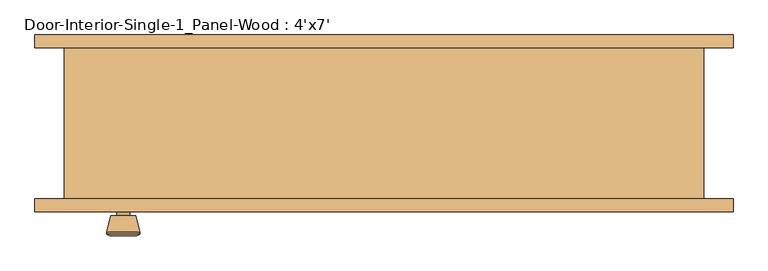
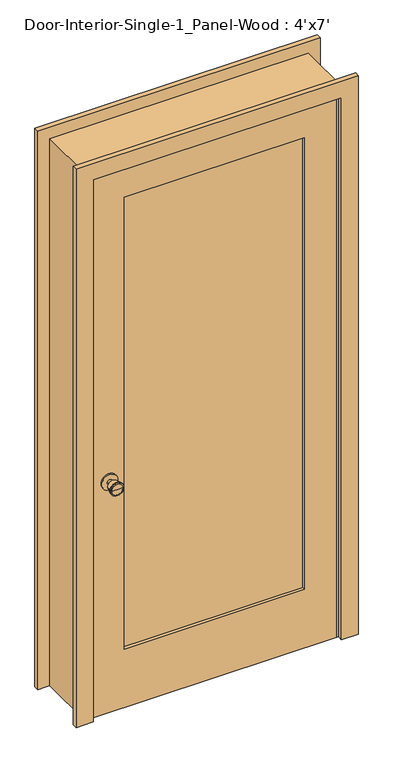
"""IFC4 building model written with IfcOpenShell, lengths in millimetres: door geometry, Door-Interior-Single-1_Panel-Wood : 4'x7'."""

from ifc_helpers import new_model, si_unit, point, frame, frame_2d, origin, place, context, project, spatial, polyline, circle_curve, trimmed, segment, composite_curve, outline, extrude, faceted_brep, source, transform, mapped, element, save
from ifc_brep_helpers import plane_surface, cylinder_surface, revolved_surface, advanced_brep


def door_interior_single_1_panel_wood_4_x7_868ee8a9(model_context):
    return source(origin(), model_context, "Body", "SolidModel", [
        advanced_brep(
        [(-393.7, -70.2, 914.4), (-403.7, -70.2, 914.4), (-383.7, -70.2, 914.4), (-373.2241324, -21.2, 914.4), (-414.1758676, -21.2, 914.4), (-393.7, -21.2, 914.4), (-368.7, -23.0278681, 914.4), (-418.7, -23.0278681, 914.4), (-368.7, -26.4915463, 914.4), (-418.7, -26.4915463, 914.4), (-375.063764, -51.2, 914.4), (-412.336236, -51.2, 914.4), (-383.7, -51.2, 914.4), (-403.7, -51.2, 914.4)],
        [
            (0, 1),
            (1, 2, circle_curve(frame((-393.7, -70.2, 914.4), z_axis=(0.0, -1.0, 0.0), x_axis=(-1.0, 0.0, 0.0)), 10.0)),
            (2, 0),
            (2, 1, circle_curve(frame((-393.7, -70.2, 914.4), z_axis=(0.0, -1.0, 0.0), x_axis=(-1.0, 0.0, 0.0)), 10.0)),
            (3, 4, circle_curve(frame((-393.7, -21.2, 914.4), z_axis=(0.0, 1.0, 0.0), x_axis=(-1.0, 0.0, 0.0)), 20.4758676)),
            (4, 5),
            (5, 3),
            (4, 3, circle_curve(frame((-393.7, -21.2, 914.4), z_axis=(0.0, 1.0, 0.0), x_axis=(-1.0, 0.0, 0.0)), 20.4758676)),
            (6, 7, circle_curve(frame((-393.7, -23.0278681, 914.4), z_axis=(0.0, 1.0, 0.0), x_axis=(-1.0, 0.0, 0.0)), 25.0)),
            (7, 4),
            (3, 6),
            (7, 6, circle_curve(frame((-393.7, -23.0278681, 914.4), z_axis=(0.0, 1.0, 0.0), x_axis=(-1.0, 0.0, 0.0)), 25.0)),
            (8, 9, circle_curve(frame((-393.7, -26.4915463, 914.4), z_axis=(0.0, 1.0, 0.0), x_axis=(-1.0, 0.0, 0.0)), 25.0)),
            (9, 7),
            (6, 8),
            (9, 8, circle_curve(frame((-393.7, -26.4915463, 914.4), z_axis=(0.0, 1.0, 0.0), x_axis=(-1.0, 0.0, 0.0)), 25.0)),
            (10, 11, circle_curve(frame((-393.7, -51.2, 914.4), z_axis=(0.0, 1.0, 0.0), x_axis=(-1.0, 0.0, 0.0)), 18.636236)),
            (11, 9),
            (8, 10),
            (11, 10, circle_curve(frame((-393.7, -51.2, 914.4), z_axis=(0.0, 1.0, 0.0), x_axis=(-1.0, 0.0, 0.0)), 18.636236)),
            (12, 13, circle_curve(frame((-393.7, -51.2, 914.4), z_axis=(0.0, 1.0, 0.0), x_axis=(-1.0, 0.0, 0.0)), 10.0)),
            (13, 11),
            (10, 12),
            (13, 12, circle_curve(frame((-393.7, -51.2, 914.4), z_axis=(0.0, 1.0, 0.0), x_axis=(-1.0, 0.0, 0.0)), 10.0)),
            (1, 13),
            (12, 2),
        ],
        [
            plane_surface(frame((-393.7, -70.2, 914.4), z_axis=(0.0, -1.0, 0.0), x_axis=(-1.0, 0.0, 0.0))),
            plane_surface(frame((-393.7, -21.2, 914.4), z_axis=(0.0, 1.0, 0.0), x_axis=(-1.0, 0.0, 0.0))),
            revolved_surface(polyline([(-414.1758676, -21.2, 914.4), (-418.7, -23.0278681, 914.4)]), (-393.7, -70.2, 914.4), (0.0, -1.0, 0.0)),
            cylinder_surface(frame((-393.7, -70.2, 914.4), z_axis=(0.0, -1.0, 0.0), x_axis=(-1.0, 0.0, 0.0)), 25.0),
            revolved_surface(polyline([(-418.7, -26.4915463, 914.4), (-412.336236, -51.2, 914.4)]), (-393.7, -70.2, 914.4), (0.0, -1.0, 0.0)),
            plane_surface(frame((-393.7, -51.2, 914.4), z_axis=(0.0, -1.0, 0.0), x_axis=(-1.0, 0.0, 0.0))),
            cylinder_surface(frame((-393.7, -70.2, 914.4), z_axis=(0.0, -1.0, 0.0), x_axis=(-1.0, 0.0, 0.0)), 10.0),
        ],
        [
            (0, [[1, 2, 3]]),
            (0, [[-3, 4, -1]]),
            (1, [[5, 6, 7]]),
            (1, [[8, -7, -6]]),
            (2, [[9, 10, -5, 11]]),
            (2, [[12, -11, -8, -10]]),
            (3, [[13, 14, -9, 15]]),
            (3, [[16, -15, -12, -14]]),
            (4, [[17, 18, -13, 19]]),
            (4, [[20, -19, -16, -18]]),
            (5, [[21, 22, -17, 23]]),
            (5, [[24, -23, -20, -22]]),
            (6, [[-2, 25, -21, 26]]),
            (6, [[-4, -26, -24, -25]]),
        ],
    ),
        extrude(outline(composite_curve([segment(trimmed(circle_curve(frame_2d((914.4, -393.7)), 30.0), [point((914.4, -423.7))], [point((914.4, -363.7))], False, "CARTESIAN"), True, "CONTINUOUS"), segment(trimmed(circle_curve(frame_2d((914.4, -393.7)), 30.0), [point((914.4, -363.7))], [point((914.4, -423.7))], False, "CARTESIAN"), True, "CONTINUOUS")], self_intersect=False)), frame((0.0, -76.2, 0.0), z_axis=(0.0, 1.0, 0.0), x_axis=(0.0, 0.0, 1.0)), (0.0, 0.0, 1.0), 6.0),
        advanced_brep(
        [(-393.7, -117.125, 914.4), (-383.7, -117.125, 914.4), (-403.7, -117.125, 914.4), (-373.2241324, -166.125, 914.4), (-393.7, -166.125, 914.4), (-414.1758676, -166.125, 914.4), (-368.7, -164.2971319, 914.4), (-418.7, -164.2971319, 914.4), (-368.7, -160.8334537, 914.4), (-418.7, -160.8334537, 914.4), (-375.063764, -136.125, 914.4), (-412.336236, -136.125, 914.4), (-383.7, -136.125, 914.4), (-403.7, -136.125, 914.4)],
        [
            (0, 1),
            (1, 2, circle_curve(frame((-393.7, -117.125, 914.4), z_axis=(0.0, 1.0, 0.0), x_axis=(-1.0, 0.0, 0.0)), 10.0)),
            (2, 0),
            (2, 1, circle_curve(frame((-393.7, -117.125, 914.4), z_axis=(0.0, 1.0, 0.0), x_axis=(-1.0, 0.0, 0.0)), 10.0)),
            (3, 4),
            (4, 5),
            (5, 3, circle_curve(frame((-393.7, -166.125, 914.4), z_axis=(0.0, -1.0, 0.0), x_axis=(-1.0, 0.0, 0.0)), 20.4758676)),
            (3, 5, circle_curve(frame((-393.7, -166.125, 914.4), z_axis=(0.0, -1.0, 0.0), x_axis=(-1.0, 0.0, 0.0)), 20.4758676)),
            (6, 3),
            (5, 7),
            (7, 6, circle_curve(frame((-393.7, -164.2971319, 914.4), z_axis=(0.0, -1.0, 0.0), x_axis=(-1.0, 0.0, 0.0)), 25.0)),
            (6, 7, circle_curve(frame((-393.7, -164.2971319, 914.4), z_axis=(0.0, -1.0, 0.0), x_axis=(-1.0, 0.0, 0.0)), 25.0)),
            (8, 6),
            (7, 9),
            (9, 8, circle_curve(frame((-393.7, -160.8334537, 914.4), z_axis=(0.0, -1.0, 0.0), x_axis=(-1.0, 0.0, 0.0)), 25.0)),
            (8, 9, circle_curve(frame((-393.7, -160.8334537, 914.4), z_axis=(0.0, -1.0, 0.0), x_axis=(-1.0, 0.0, 0.0)), 25.0)),
            (10, 8),
            (9, 11),
            (11, 10, circle_curve(frame((-393.7, -136.125, 914.4), z_axis=(0.0, -1.0, 0.0), x_axis=(-1.0, 0.0, 0.0)), 18.636236)),
            (10, 11, circle_curve(frame((-393.7, -136.125, 914.4), z_axis=(0.0, -1.0, 0.0), x_axis=(-1.0, 0.0, 0.0)), 18.636236)),
            (12, 10),
            (11, 13),
            (13, 12, circle_curve(frame((-393.7, -136.125, 914.4), z_axis=(0.0, -1.0, 0.0), x_axis=(-1.0, 0.0, 0.0)), 10.0)),
            (12, 13, circle_curve(frame((-393.7, -136.125, 914.4), z_axis=(0.0, -1.0, 0.0), x_axis=(-1.0, 0.0, 0.0)), 10.0)),
            (1, 12),
            (13, 2),
        ],
        [
            plane_surface(frame((-393.7, -117.125, 914.4), z_axis=(0.0, 1.0, 0.0), x_axis=(-1.0, 0.0, 0.0))),
            plane_surface(frame((-393.7, -166.125, 914.4), z_axis=(0.0, -1.0, 0.0), x_axis=(-1.0, 0.0, 0.0))),
            revolved_surface(polyline([(-414.1758676, -166.125, 914.4), (-418.7, -164.2971319, 914.4)]), (-393.7, -117.125, 914.4), (0.0, 1.0, 0.0)),
            cylinder_surface(frame((-393.7, -117.125, 914.4), z_axis=(0.0, 1.0, 0.0), x_axis=(-1.0, 0.0, 0.0)), 25.0),
            revolved_surface(polyline([(-418.7, -160.8334537, 914.4), (-412.336236, -136.125, 914.4)]), (-393.7, -117.125, 914.4), (0.0, 1.0, 0.0)),
            plane_surface(frame((-393.7, -136.125, 914.4), z_axis=(0.0, 1.0, 0.0), x_axis=(-1.0, 0.0, 0.0))),
            cylinder_surface(frame((-393.7, -117.125, 914.4), z_axis=(0.0, 1.0, 0.0), x_axis=(-1.0, 0.0, 0.0)), 10.0),
        ],
        [
            (0, [[1, 2, 3]]),
            (0, [[-3, 4, -1]]),
            (1, [[5, 6, 7]]),
            (1, [[-6, -5, 8]]),
            (2, [[9, -7, 10, 11]]),
            (2, [[-10, -8, -9, 12]]),
            (3, [[13, -11, 14, 15]]),
            (3, [[-14, -12, -13, 16]]),
            (4, [[17, -15, 18, 19]]),
            (4, [[-18, -16, -17, 20]]),
            (5, [[21, -19, 22, 23]]),
            (5, [[-22, -20, -21, 24]]),
            (6, [[25, -23, 26, -2]]),
            (6, [[-26, -24, -25, -4]]),
        ],
    ),
        extrude(outline(composite_curve([segment(trimmed(circle_curve(frame_2d((914.4, -393.7)), 30.0), [point((914.4, -423.7))], [point((914.4, -363.7))], False, "CARTESIAN"), True, "CONTINUOUS"), segment(trimmed(circle_curve(frame_2d((914.4, -393.7)), 30.0), [point((914.4, -363.7))], [point((914.4, -423.7))], False, "CARTESIAN"), True, "CONTINUOUS")], self_intersect=False)), frame((0.0, -117.125, 0.0), z_axis=(0.0, 1.0, 0.0), x_axis=(0.0, 0.0, 1.0)), (0.0, 0.0, 1.0), 6.0),
        faceted_brep([(482.6, -111.125, 0.0), (457.2, -111.125, 0.0), (457.2, -76.2, 0.0), (444.5, -76.2, 0.0), (444.5, -41.275, 0.0), (457.2, -41.275, 0.0), (457.2, 117.475, 0.0), (482.6, 117.475, 0.0), (482.6, 117.475, 2159.0), (482.6, -111.125, 2159.0), (457.2, 117.475, 2133.6), (-457.2, 117.475, 2133.6), (-457.2, 117.475, 0.0), (-482.6, 117.475, 0.0), (-482.6, 117.475, 2159.0), (457.2, -41.275, 2133.6), (444.5, -41.275, 2120.9), (-444.5, -41.275, 2120.9), (-444.5, -41.275, 0.0), (-457.2, -41.275, 0.0), (-457.2, -41.275, 2133.6), (444.5, -76.2, 2120.9), (457.2, -76.2, 2133.6), (-457.2, -76.2, 2133.6), (-457.2, -76.2, 0.0), (-444.5, -76.2, 0.0), (-444.5, -76.2, 2120.9), (457.2, -111.125, 2133.6), (-482.6, -111.125, 2159.0), (-482.6, -111.125, 0.0), (-457.2, -111.125, 0.0), (-457.2, -111.125, 2133.6)], [[[0, 1, 2, 3, 4, 5, 6, 7]], [[7, 8, 9, 0]], [[6, 10, 11, 12, 13, 14, 8, 7]], [[5, 15, 10, 6]], [[4, 16, 17, 18, 19, 20, 15, 5]], [[3, 21, 16, 4]], [[2, 22, 23, 24, 25, 26, 21, 3]], [[1, 27, 22, 2]], [[0, 9, 28, 29, 30, 31, 27, 1]], [[8, 14, 28, 9]], [[15, 20, 11, 10]], [[21, 26, 17, 16]], [[27, 31, 23, 22]], [[29, 13, 12, 19, 18, 25, 24, 30]], [[14, 13, 29, 28]], [[20, 19, 12, 11]], [[26, 25, 18, 17]], [[31, 30, 24, 23]]]),
        extrude(outline(polyline([(2133.6, -457.2), (0.0, -457.2), (0.0, 457.2), (2133.6, 457.2), (2133.6, -457.2)]), holes=[polyline([(2014.5375, -336.55), (2014.5375, 336.55), (231.775, 336.55), (231.775, -336.55), (2014.5375, -336.55)])]), frame((0.0, -111.125, 0.0), z_axis=(0.0, 1.0, 0.0), x_axis=(0.0, 0.0, 1.0)), (0.0, 0.0, 1.0), 34.925),
        extrude(outline(polyline([(336.55, -87.8416667), (336.55, -99.4833333), (-336.55, -99.4833333), (-336.55, -87.8416667), (336.55, -87.8416667)])), frame((0.0, 0.0, 231.775), z_axis=(0.0, 0.0, 1.0), x_axis=(1.0, 0.0, 0.0)), (0.0, 0.0, 1.0), 1782.7625),
        extrude(outline(polyline([(0.0, 527.05), (2203.45, 527.05), (2203.45, -527.05), (0.0, -527.05), (0.0, -463.55), (2139.95, -463.55), (2139.95, 463.55), (0.0, 463.55), (0.0, 527.05)])), frame((0.0, -130.175, 0.0), z_axis=(0.0, 1.0, 0.0), x_axis=(0.0, 0.0, 1.0)), (0.0, 0.0, 1.0), 19.05),
        extrude(outline(polyline([(0.0, 527.05), (2203.45, 527.05), (2203.45, -527.05), (0.0, -527.05), (0.0, -463.55), (2139.95, -463.55), (2139.95, 463.55), (0.0, 463.55), (0.0, 527.05)])), frame((0.0, 117.475, 0.0), z_axis=(0.0, 1.0, 0.0), x_axis=(0.0, 0.0, 1.0)), (0.0, 0.0, 1.0), 19.05),
    ])


if __name__ == "__main__":
    model = new_model("IFC4")
    model_context = context("Model", 3, world=origin())
    ifc_project = project(units=[si_unit("LENGTHUNIT", "METRE", prefix="MILLI")], contexts=[model_context])
    site = spatial("IfcSite", under=ifc_project)
    building = spatial("IfcBuilding", under=site)
    placement = place(None, origin())
    door_interior_single_1_panel_wood_4_x7_shape = door_interior_single_1_panel_wood_4_x7_868ee8a9(model_context)
    element("IfcDoor", 1, ObjectType="Door-Interior-Single-1_Panel-Wood : 4'x7'", at=placement, inside=building, context=model_context, shape_type="MappedRepresentation", body=[
        mapped(door_interior_single_1_panel_wood_4_x7_shape, transform((0.0, 0.0, 0.0), x_axis=(1.0, 0.0, 0.0), y_axis=(0.0, 1.0, 0.0), z_axis=(0.0, 0.0, 1.0))),
    ])
    save(model, "model.ifc")

# Revit data of these elements
# Type "Door-Interior-Single-1_Panel-Wood : 4'x7'"
#   Type Mark = "9"
#   Assembly Code = "C1020300"
#   Analytic Construction = "Wooden"
#   Top Rail = 0' - 4 11/16"
#   Thickness = 0' - 1 3/8"
#   Thermal Resistance (R) = 2.5876 (h·ft²·°F)/BTU
#   Swing Angle [instance default] = 90.00°
#   Stiles = 0' - 4 3/4"
#   Rough Width = 3' - 2"
#   Rough Height = 7' - 1"
#   Height = 7' - 0"
#   Width = 3' - 0"
#   Heat Transfer Coefficient (U) = 0.3865 BTU/(h·ft²·°F)
#   Bottom Rail = 0' - 9 1/8"
#   Trim Material = Cherry
#   Panel Material = Cherry
#   Frame Material = Cherry
#   Door Handle Material = Aluminum
#   Visual Light Transmittance = 0
#   Solar Heat Gain Coefficient = 0
#   Wall Closure = (empty or 0)
#   Function = (empty or 0)
# Element 1 (IfcDoor, "Door-Interior-Single-1_Panel-Wood : 4'x7'")
#   Materials on its faces: "Cherry", "Aluminum"
# Materials
#   "Cherry": class "Wood", colour RGB 226 177 128, transparency 0, Description = "Prunus Serotina", Cost = 0
#   "Aluminum": class "Metal", colour RGB 247 247 247, transparency 0, Description = "Aluminum 6061", Cost = 0
